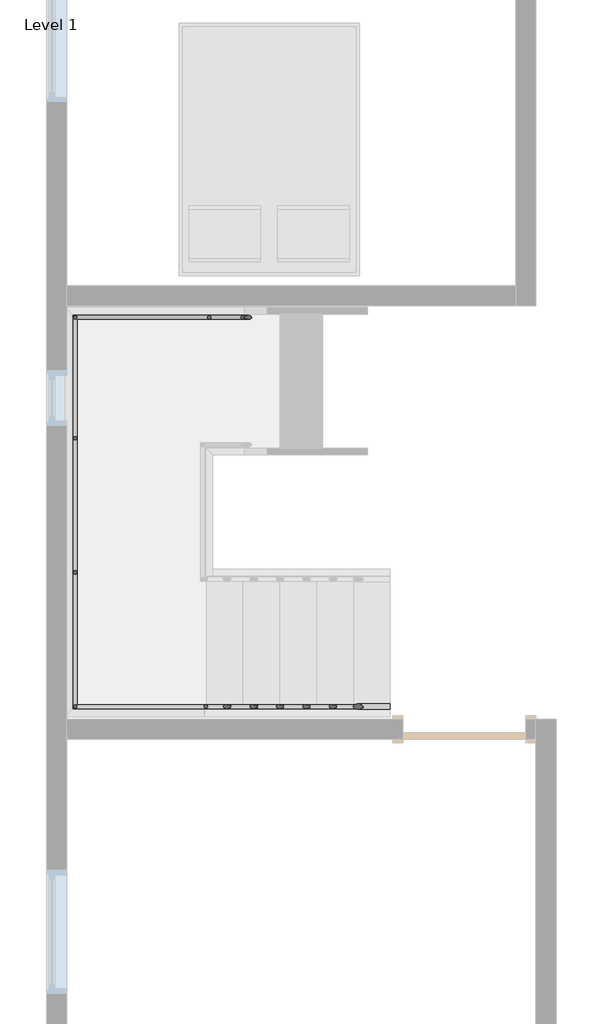
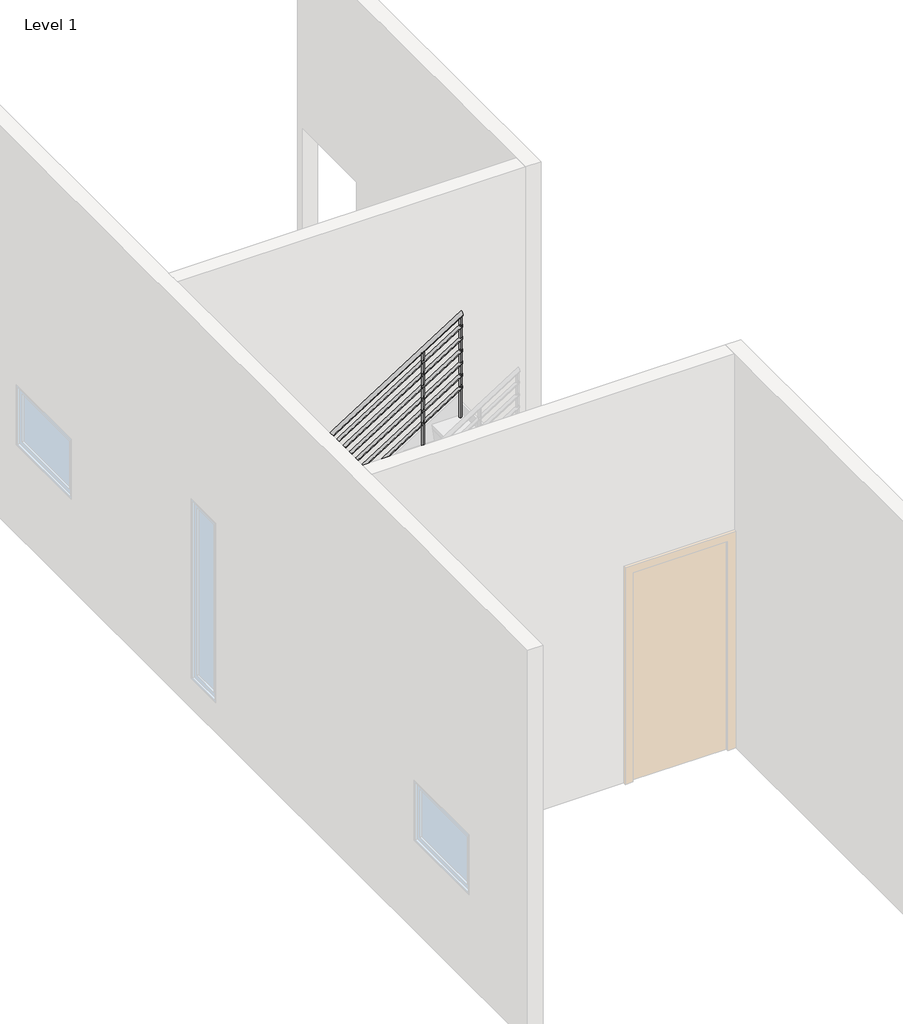
# One storey, part 3 of 4: 1 railing.
"""IFC4 building model written with IfcOpenShell, lengths in millimetres."""

from ifc_helpers import new_model, si_unit, point, frame, frame_2d, origin, place, context, project, spatial, circle_curve, ellipse_curve, trimmed, segment, composite_curve, outline, extrude, element, save
from ifc_brep_helpers import plane_surface, cylinder_surface, advanced_brep

model = new_model("IFC4")

# Units and contexts
model_context = context("Model", 3, world=origin())
ifc_project = project(units=[si_unit("LENGTHUNIT", "METRE", prefix="MILLI")], contexts=[model_context])

# Site, building, storey
site = spatial("IfcSite", under=ifc_project)
building = spatial("IfcBuilding", under=site)
storey = spatial("IfcBuildingStorey", under=building, Name="Level 1", Elevation=0.0)

# Railing
placement = place(None, origin())
element("IfcRailing", 1, ObjectType="900mm Pipe", at=placement, inside=storey, context=model_context, shape_type="SolidModel", body=[
    advanced_brep(
    [(-10589.1151057, 893.2798105, 1050.2491997), (-10589.1151057, 853.2798105, 1050.2491997), (-11969.9085587, 893.2798105, 1923.4782609), (-11969.9085587, 853.2798105, 1923.4782609), (-12918.740887, 893.2798105, 1923.4782609), (-12958.740887, 853.2798105, 1923.4782609), (-12918.740887, 3754.7656289, 1923.4782609), (-12958.740887, 3794.7656289, 1923.4782609), (-11683.3216527, 3754.7656289, 1923.4782609), (-11683.3216527, 3794.7656289, 1923.4782609), (-10314.1151057, 3754.7656289, 2789.3796345), (-10314.1151057, 3794.7656289, 2789.3796345)],
    [
        (0, 1, ellipse_curve(frame((-10589.1151057, 873.2798105, 1050.2491997), z_axis=(1.0, 0.0, 0.0), x_axis=(0.0, 0.0, -1.0)), 23.6638438, 20.0)),
        (1, 0, ellipse_curve(frame((-10589.1151057, 873.2798105, 1050.2491997), z_axis=(1.0, 0.0, 0.0), x_axis=(0.0, 0.0, -1.0)), 23.6638438, 20.0)),
        (0, 2),
        (2, 3, ellipse_curve(frame((-11969.9085587, 873.2798105, 1923.4782609), z_axis=(0.9605132043335071, 0.0, -0.27823440531497595), x_axis=(-0.2782344053149755, 0.0, -0.9605132043335074)), 20.822202, 20.0)),
        (3, 1),
        (3, 2, ellipse_curve(frame((-11969.9085587, 873.2798105, 1923.4782609), z_axis=(0.9605132043335071, 0.0, -0.27823440531497595), x_axis=(-0.2782344053149755, 0.0, -0.9605132043335074)), 20.822202, 20.0)),
        (2, 4),
        (4, 5, ellipse_curve(frame((-12938.740887, 873.2798105, 1923.4782609), z_axis=(0.7071067811865439, -0.7071067811865511, 0.0), x_axis=(0.7071067811865511, 0.7071067811865439, 0.0)), 28.2842712, 20.0)),
        (5, 3),
        (5, 4, ellipse_curve(frame((-12938.740887, 873.2798105, 1923.4782609), z_axis=(0.7071067811865439, -0.7071067811865511, 0.0), x_axis=(0.7071067811865511, 0.7071067811865439, 0.0)), 28.2842712, 20.0)),
        (4, 6),
        (6, 7, ellipse_curve(frame((-12938.740887, 3774.7656289, 1923.4782609), z_axis=(-0.7071067811865511, -0.7071067811865439, 0.0), x_axis=(0.7071067811865439, -0.7071067811865512, 0.0)), 28.2842712, 20.0)),
        (7, 5),
        (7, 6, ellipse_curve(frame((-12938.740887, 3774.7656289, 1923.4782609), z_axis=(-0.7071067811865511, -0.7071067811865439, 0.0), x_axis=(0.7071067811865439, -0.7071067811865512, 0.0)), 28.2842712, 20.0)),
        (6, 8),
        (8, 9, ellipse_curve(frame((-11683.3216527, 3774.7656289, 1923.4782609), z_axis=(-0.9605132043335074, 0.0, -0.2782344053149752), x_axis=(-0.2782344053149752, 0.0, 0.9605132043335074)), 20.822202, 20.0)),
        (9, 7),
        (9, 8, ellipse_curve(frame((-11683.3216527, 3774.7656289, 1923.4782609), z_axis=(-0.9605132043335074, 0.0, -0.2782344053149752), x_axis=(-0.2782344053149752, 0.0, 0.9605132043335074)), 20.822202, 20.0)),
        (10, 11, ellipse_curve(frame((-10314.1151057, 3774.7656289, 2789.3796345), z_axis=(1.0, 0.0, 0.0), x_axis=(0.0, 0.0, -1.0)), 23.6638438, 20.0)),
        (11, 10, ellipse_curve(frame((-10314.1151057, 3774.7656289, 2789.3796345), z_axis=(1.0, 0.0, 0.0), x_axis=(0.0, 0.0, -1.0)), 23.6638438, 20.0)),
        (8, 10),
        (11, 9),
    ],
    [
        plane_surface(frame((-10589.1151057, 873.2798105, 1073.9130435), z_axis=(1.0, 0.0, 0.0), x_axis=(0.0, -1.0, 0.0))),
        cylinder_surface(frame((-10599.8050185, 873.2798105, 1057.0096189), z_axis=(0.8451712313980434, 0.0, -0.5344956404098309), x_axis=(0.0, -1.0, 0.0)), 20.0),
        cylinder_surface(frame((-11964.1151057, 873.2798105, 1923.4782609), z_axis=(1.0, 0.0, 0.0), x_axis=(0.0, -1.0, 0.0)), 20.0),
        cylinder_surface(frame((-12938.740887, 873.2798105, 1923.4782609), z_axis=(0.0, -1.0, 0.0), x_axis=(-1.0, 0.0, 0.0)), 20.0),
        cylinder_surface(frame((-12938.740887, 3774.7656289, 1923.4782609), z_axis=(-1.0, 0.0, 0.0), x_axis=(0.0, 1.0, 0.0)), 20.0),
        plane_surface(frame((-10314.1151057, 3774.7656289, 2813.0434783), z_axis=(1.0, 0.0, 0.0), x_axis=(0.0, 1.0, 0.0))),
        cylinder_surface(frame((-11678.4251929, 3774.7656289, 1926.5748362), z_axis=(-0.8451712313980442, 0.0, -0.5344956404098294), x_axis=(0.0, 1.0, 0.0)), 20.0),
    ],
    [
        (0, [[1, 2]]),
        (1, [[-1, 3, 4, 5]]),
        (1, [[-2, -5, 6, -3]]),
        (2, [[-4, 7, 8, 9]]),
        (2, [[-6, -9, 10, -7]]),
        (3, [[-8, 11, 12, 13]]),
        (3, [[-10, -13, 14, -11]]),
        (4, [[-12, 15, 16, 17]]),
        (4, [[-14, -17, 18, -15]]),
        (5, [[19, 20]]),
        (6, [[-16, 21, -20, 22]]),
        (6, [[-18, -22, -19, -21]]),
    ],
),
    advanced_brep(
    [(-10589.1151057, 888.2798105, 931.1651606), (-10589.1151057, 858.2798105, 931.1651606), (-11968.4601955, 888.2798105, 1803.4782609), (-11968.4601955, 858.2798105, 1803.4782609), (-12923.740887, 888.2798105, 1803.4782609), (-12953.740887, 858.2798105, 1803.4782609), (-12923.740887, 3759.7656289, 1803.4782609), (-12953.740887, 3789.7656289, 1803.4782609), (-11684.7700159, 3759.7656289, 1803.4782609), (-11684.7700159, 3789.7656289, 1803.4782609), (-10314.1151057, 3759.7656289, 2670.2955954), (-10314.1151057, 3789.7656289, 2670.2955954)],
    [
        (0, 1, ellipse_curve(frame((-10589.1151057, 873.2798105, 931.1651606), z_axis=(1.0, 0.0, 0.0), x_axis=(0.0, 0.0, -1.0)), 17.7478828, 15.0)),
        (1, 0, ellipse_curve(frame((-10589.1151057, 873.2798105, 931.1651606), z_axis=(1.0, 0.0, 0.0), x_axis=(0.0, 0.0, -1.0)), 17.7478828, 15.0)),
        (0, 2),
        (2, 3, ellipse_curve(frame((-11968.4601955, 873.2798105, 1803.4782609), z_axis=(0.9605132043335071, 0.0, -0.2782344053149759), x_axis=(-0.27823440531497556, 0.0, -0.9605132043335073)), 15.6166515, 15.0)),
        (3, 1),
        (3, 2, ellipse_curve(frame((-11968.4601955, 873.2798105, 1803.4782609), z_axis=(0.9605132043335071, 0.0, -0.2782344053149759), x_axis=(-0.27823440531497556, 0.0, -0.9605132043335073)), 15.6166515, 15.0)),
        (2, 4),
        (4, 5, ellipse_curve(frame((-12938.740887, 873.2798105, 1803.4782609), z_axis=(0.7071067811865439, -0.7071067811865511, 0.0), x_axis=(0.7071067811865511, 0.7071067811865439, 0.0)), 21.2132034, 15.0)),
        (5, 3),
        (5, 4, ellipse_curve(frame((-12938.740887, 873.2798105, 1803.4782609), z_axis=(0.7071067811865439, -0.7071067811865511, 0.0), x_axis=(0.7071067811865511, 0.7071067811865439, 0.0)), 21.2132034, 15.0)),
        (4, 6),
        (6, 7, ellipse_curve(frame((-12938.740887, 3774.7656289, 1803.4782609), z_axis=(-0.7071067811865511, -0.7071067811865439, 0.0), x_axis=(0.7071067811865439, -0.7071067811865512, 0.0)), 21.2132034, 15.0)),
        (7, 5),
        (7, 6, ellipse_curve(frame((-12938.740887, 3774.7656289, 1803.4782609), z_axis=(-0.7071067811865511, -0.7071067811865439, 0.0), x_axis=(0.7071067811865439, -0.7071067811865512, 0.0)), 21.2132034, 15.0)),
        (6, 8),
        (8, 9, ellipse_curve(frame((-11684.7700159, 3774.7656289, 1803.4782609), z_axis=(-0.9605132043335073, 0.0, -0.2782344053149753), x_axis=(-0.2782344053149759, 0.0, 0.9605132043335072)), 15.6166515, 15.0)),
        (9, 7),
        (9, 8, ellipse_curve(frame((-11684.7700159, 3774.7656289, 1803.4782609), z_axis=(-0.9605132043335073, 0.0, -0.2782344053149753), x_axis=(-0.2782344053149759, 0.0, 0.9605132043335072)), 15.6166515, 15.0)),
        (10, 11, ellipse_curve(frame((-10314.1151057, 3774.7656289, 2670.2955954), z_axis=(1.0, 0.0, 0.0), x_axis=(0.0, 0.0, -1.0)), 17.7478828, 15.0)),
        (11, 10, ellipse_curve(frame((-10314.1151057, 3774.7656289, 2670.2955954), z_axis=(1.0, 0.0, 0.0), x_axis=(0.0, 0.0, -1.0)), 17.7478828, 15.0)),
        (8, 10),
        (11, 9),
    ],
    [
        plane_surface(frame((-10589.1151057, 873.2798105, 948.9130435), z_axis=(1.0, 0.0, 0.0), x_axis=(0.0, -1.0, 0.0))),
        cylinder_surface(frame((-10597.1325403, 873.2798105, 936.235475), z_axis=(0.8451712313980434, 0.0, -0.5344956404098308), x_axis=(0.0, -1.0, 0.0)), 15.0),
        cylinder_surface(frame((-11964.1151057, 873.2798105, 1803.4782609), z_axis=(1.0, 0.0, 0.0), x_axis=(0.0, -1.0, 0.0)), 15.0),
        cylinder_surface(frame((-12938.740887, 873.2798105, 1803.4782609), z_axis=(0.0, -1.0, 0.0), x_axis=(-1.0, 0.0, 0.0)), 15.0),
        cylinder_surface(frame((-12938.740887, 3774.7656289, 1803.4782609), z_axis=(-1.0, 0.0, 0.0), x_axis=(0.0, 1.0, 0.0)), 15.0),
        plane_surface(frame((-10314.1151057, 3774.7656289, 2688.0434783), z_axis=(1.0, 0.0, 0.0), x_axis=(0.0, 1.0, 0.0))),
        cylinder_surface(frame((-11681.0976711, 3774.7656289, 1805.8006924), z_axis=(-0.845171231398044, 0.0, -0.5344956404098297), x_axis=(0.0, 1.0, 0.0)), 15.0),
    ],
    [
        (0, [[1, 2]]),
        (1, [[-1, 3, 4, 5]]),
        (1, [[-2, -5, 6, -3]]),
        (2, [[-4, 7, 8, 9]]),
        (2, [[-6, -9, 10, -7]]),
        (3, [[-8, 11, 12, 13]]),
        (3, [[-10, -13, 14, -11]]),
        (4, [[-12, 15, 16, 17]]),
        (4, [[-14, -17, 18, -15]]),
        (5, [[19, 20]]),
        (6, [[-16, 21, -20, 22]]),
        (6, [[-18, -22, -19, -21]]),
    ],
),
    advanced_brep(
    [(-10589.1151057, 888.2798105, 806.1651606), (-10589.1151057, 858.2798105, 806.1651606), (-11968.4601955, 888.2798105, 1678.4782609), (-11968.4601955, 858.2798105, 1678.4782609), (-12923.740887, 888.2798105, 1678.4782609), (-12953.740887, 858.2798105, 1678.4782609), (-12923.740887, 3759.7656289, 1678.4782609), (-12953.740887, 3789.7656289, 1678.4782609), (-11684.7700159, 3759.7656289, 1678.4782609), (-11684.7700159, 3789.7656289, 1678.4782609), (-10314.1151057, 3759.7656289, 2545.2955954), (-10314.1151057, 3789.7656289, 2545.2955954)],
    [
        (0, 1, ellipse_curve(frame((-10589.1151057, 873.2798105, 806.1651606), z_axis=(1.0, 0.0, 0.0), x_axis=(0.0, 0.0, -1.0)), 17.7478828, 15.0)),
        (1, 0, ellipse_curve(frame((-10589.1151057, 873.2798105, 806.1651606), z_axis=(1.0, 0.0, 0.0), x_axis=(0.0, 0.0, -1.0)), 17.7478828, 15.0)),
        (0, 2),
        (2, 3, ellipse_curve(frame((-11968.4601955, 873.2798105, 1678.4782609), z_axis=(0.9605132043335071, 0.0, -0.2782344053149759), x_axis=(-0.27823440531497556, 0.0, -0.9605132043335073)), 15.6166515, 15.0)),
        (3, 1),
        (3, 2, ellipse_curve(frame((-11968.4601955, 873.2798105, 1678.4782609), z_axis=(0.9605132043335071, 0.0, -0.2782344053149759), x_axis=(-0.27823440531497556, 0.0, -0.9605132043335073)), 15.6166515, 15.0)),
        (2, 4),
        (4, 5, ellipse_curve(frame((-12938.740887, 873.2798105, 1678.4782609), z_axis=(0.7071067811865439, -0.7071067811865511, 0.0), x_axis=(0.7071067811865511, 0.7071067811865439, 0.0)), 21.2132034, 15.0)),
        (5, 3),
        (5, 4, ellipse_curve(frame((-12938.740887, 873.2798105, 1678.4782609), z_axis=(0.7071067811865439, -0.7071067811865511, 0.0), x_axis=(0.7071067811865511, 0.7071067811865439, 0.0)), 21.2132034, 15.0)),
        (4, 6),
        (6, 7, ellipse_curve(frame((-12938.740887, 3774.7656289, 1678.4782609), z_axis=(-0.7071067811865511, -0.7071067811865439, 0.0), x_axis=(0.7071067811865439, -0.7071067811865512, 0.0)), 21.2132034, 15.0)),
        (7, 5),
        (7, 6, ellipse_curve(frame((-12938.740887, 3774.7656289, 1678.4782609), z_axis=(-0.7071067811865511, -0.7071067811865439, 0.0), x_axis=(0.7071067811865439, -0.7071067811865512, 0.0)), 21.2132034, 15.0)),
        (6, 8),
        (8, 9, ellipse_curve(frame((-11684.7700159, 3774.7656289, 1678.4782609), z_axis=(-0.9605132043335073, 0.0, -0.27823440531497523), x_axis=(-0.27823440531497595, 0.0, 0.9605132043335072)), 15.6166515, 15.0)),
        (9, 7),
        (9, 8, ellipse_curve(frame((-11684.7700159, 3774.7656289, 1678.4782609), z_axis=(-0.9605132043335073, 0.0, -0.27823440531497523), x_axis=(-0.27823440531497595, 0.0, 0.9605132043335072)), 15.6166515, 15.0)),
        (10, 11, ellipse_curve(frame((-10314.1151057, 3774.7656289, 2545.2955954), z_axis=(1.0, 0.0, 0.0), x_axis=(0.0, 0.0, -1.0)), 17.7478828, 15.0)),
        (11, 10, ellipse_curve(frame((-10314.1151057, 3774.7656289, 2545.2955954), z_axis=(1.0, 0.0, 0.0), x_axis=(0.0, 0.0, -1.0)), 17.7478828, 15.0)),
        (8, 10),
        (11, 9),
    ],
    [
        plane_surface(frame((-10589.1151057, 873.2798105, 823.9130435), z_axis=(1.0, 0.0, 0.0), x_axis=(0.0, -1.0, 0.0))),
        cylinder_surface(frame((-10597.1325403, 873.2798105, 811.235475), z_axis=(0.8451712313980434, 0.0, -0.5344956404098308), x_axis=(0.0, -1.0, 0.0)), 15.0),
        cylinder_surface(frame((-11964.1151057, 873.2798105, 1678.4782609), z_axis=(1.0, 0.0, 0.0), x_axis=(0.0, -1.0, 0.0)), 15.0),
        cylinder_surface(frame((-12938.740887, 873.2798105, 1678.4782609), z_axis=(0.0, -1.0, 0.0), x_axis=(-1.0, 0.0, 0.0)), 15.0),
        cylinder_surface(frame((-12938.740887, 3774.7656289, 1678.4782609), z_axis=(-1.0, 0.0, 0.0), x_axis=(0.0, 1.0, 0.0)), 15.0),
        plane_surface(frame((-10314.1151057, 3774.7656289, 2563.0434783), z_axis=(1.0, 0.0, 0.0), x_axis=(0.0, 1.0, 0.0))),
        cylinder_surface(frame((-11681.0976711, 3774.7656289, 1680.8006924), z_axis=(-0.8451712313980441, 0.0, -0.5344956404098296), x_axis=(0.0, 1.0, 0.0)), 15.0),
    ],
    [
        (0, [[1, 2]]),
        (1, [[-1, 3, 4, 5]]),
        (1, [[-2, -5, 6, -3]]),
        (2, [[-4, 7, 8, 9]]),
        (2, [[-6, -9, 10, -7]]),
        (3, [[-8, 11, 12, 13]]),
        (3, [[-10, -13, 14, -11]]),
        (4, [[-12, 15, 16, 17]]),
        (4, [[-14, -17, 18, -15]]),
        (5, [[19, 20]]),
        (6, [[-16, 21, -20, 22]]),
        (6, [[-18, -22, -19, -21]]),
    ],
),
    advanced_brep(
    [(-10589.1151057, 888.2798105, 681.1651606), (-10589.1151057, 858.2798105, 681.1651606), (-11968.4601955, 888.2798105, 1553.4782609), (-11968.4601955, 858.2798105, 1553.4782609), (-12923.740887, 888.2798105, 1553.4782609), (-12953.740887, 858.2798105, 1553.4782609), (-12923.740887, 3759.7656289, 1553.4782609), (-12953.740887, 3789.7656289, 1553.4782609), (-11684.7700159, 3759.7656289, 1553.4782609), (-11684.7700159, 3789.7656289, 1553.4782609), (-10314.1151057, 3759.7656289, 2420.2955954), (-10314.1151057, 3789.7656289, 2420.2955954)],
    [
        (0, 1, ellipse_curve(frame((-10589.1151057, 873.2798105, 681.1651606), z_axis=(1.0, 0.0, 0.0), x_axis=(0.0, 0.0, -1.0)), 17.7478828, 15.0)),
        (1, 0, ellipse_curve(frame((-10589.1151057, 873.2798105, 681.1651606), z_axis=(1.0, 0.0, 0.0), x_axis=(0.0, 0.0, -1.0)), 17.7478828, 15.0)),
        (0, 2),
        (2, 3, ellipse_curve(frame((-11968.4601955, 873.2798105, 1553.4782609), z_axis=(0.9605132043335071, 0.0, -0.2782344053149759), x_axis=(-0.27823440531497556, 0.0, -0.9605132043335073)), 15.6166515, 15.0)),
        (3, 1),
        (3, 2, ellipse_curve(frame((-11968.4601955, 873.2798105, 1553.4782609), z_axis=(0.9605132043335071, 0.0, -0.2782344053149759), x_axis=(-0.27823440531497556, 0.0, -0.9605132043335073)), 15.6166515, 15.0)),
        (2, 4),
        (4, 5, ellipse_curve(frame((-12938.740887, 873.2798105, 1553.4782609), z_axis=(0.7071067811865439, -0.7071067811865511, 0.0), x_axis=(0.7071067811865511, 0.7071067811865439, 0.0)), 21.2132034, 15.0)),
        (5, 3),
        (5, 4, ellipse_curve(frame((-12938.740887, 873.2798105, 1553.4782609), z_axis=(0.7071067811865439, -0.7071067811865511, 0.0), x_axis=(0.7071067811865511, 0.7071067811865439, 0.0)), 21.2132034, 15.0)),
        (4, 6),
        (6, 7, ellipse_curve(frame((-12938.740887, 3774.7656289, 1553.4782609), z_axis=(-0.7071067811865511, -0.7071067811865439, 0.0), x_axis=(0.7071067811865439, -0.7071067811865512, 0.0)), 21.2132034, 15.0)),
        (7, 5),
        (7, 6, ellipse_curve(frame((-12938.740887, 3774.7656289, 1553.4782609), z_axis=(-0.7071067811865511, -0.7071067811865439, 0.0), x_axis=(0.7071067811865439, -0.7071067811865512, 0.0)), 21.2132034, 15.0)),
        (6, 8),
        (8, 9, ellipse_curve(frame((-11684.7700159, 3774.7656289, 1553.4782609), z_axis=(-0.9605132043335073, 0.0, -0.2782344053149753), x_axis=(-0.2782344053149759, 0.0, 0.9605132043335072)), 15.6166515, 15.0)),
        (9, 7),
        (9, 8, ellipse_curve(frame((-11684.7700159, 3774.7656289, 1553.4782609), z_axis=(-0.9605132043335073, 0.0, -0.2782344053149753), x_axis=(-0.2782344053149759, 0.0, 0.9605132043335072)), 15.6166515, 15.0)),
        (10, 11, ellipse_curve(frame((-10314.1151057, 3774.7656289, 2420.2955954), z_axis=(1.0, 0.0, 0.0), x_axis=(0.0, 0.0, -1.0)), 17.7478828, 15.0)),
        (11, 10, ellipse_curve(frame((-10314.1151057, 3774.7656289, 2420.2955954), z_axis=(1.0, 0.0, 0.0), x_axis=(0.0, 0.0, -1.0)), 17.7478828, 15.0)),
        (8, 10),
        (11, 9),
    ],
    [
        plane_surface(frame((-10589.1151057, 873.2798105, 698.9130435), z_axis=(1.0, 0.0, 0.0), x_axis=(0.0, -1.0, 0.0))),
        cylinder_surface(frame((-10597.1325403, 873.2798105, 686.235475), z_axis=(0.8451712313980434, 0.0, -0.5344956404098308), x_axis=(0.0, -1.0, 0.0)), 15.0),
        cylinder_surface(frame((-11964.1151057, 873.2798105, 1553.4782609), z_axis=(1.0, 0.0, 0.0), x_axis=(0.0, -1.0, 0.0)), 15.0),
        cylinder_surface(frame((-12938.740887, 873.2798105, 1553.4782609), z_axis=(0.0, -1.0, 0.0), x_axis=(-1.0, 0.0, 0.0)), 15.0),
        cylinder_surface(frame((-12938.740887, 3774.7656289, 1553.4782609), z_axis=(-1.0, 0.0, 0.0), x_axis=(0.0, 1.0, 0.0)), 15.0),
        plane_surface(frame((-10314.1151057, 3774.7656289, 2438.0434783), z_axis=(1.0, 0.0, 0.0), x_axis=(0.0, 1.0, 0.0))),
        cylinder_surface(frame((-11681.0976711, 3774.7656289, 1555.8006924), z_axis=(-0.845171231398044, 0.0, -0.5344956404098297), x_axis=(0.0, 1.0, 0.0)), 15.0),
    ],
    [
        (0, [[1, 2]]),
        (1, [[-1, 3, 4, 5]]),
        (1, [[-2, -5, 6, -3]]),
        (2, [[-4, 7, 8, 9]]),
        (2, [[-6, -9, 10, -7]]),
        (3, [[-8, 11, 12, 13]]),
        (3, [[-10, -13, 14, -11]]),
        (4, [[-12, 15, 16, 17]]),
        (4, [[-14, -17, 18, -15]]),
        (5, [[19, 20]]),
        (6, [[-16, 21, -20, 22]]),
        (6, [[-18, -22, -19, -21]]),
    ],
),
    advanced_brep(
    [(-10589.1151057, 888.2798105, 556.1651606), (-10589.1151057, 858.2798105, 556.1651606), (-11968.4601955, 888.2798105, 1428.4782609), (-11968.4601955, 858.2798105, 1428.4782609), (-12923.740887, 888.2798105, 1428.4782609), (-12953.740887, 858.2798105, 1428.4782609), (-12923.740887, 3759.7656289, 1428.4782609), (-12953.740887, 3789.7656289, 1428.4782609), (-11684.7700159, 3759.7656289, 1428.4782609), (-11684.7700159, 3789.7656289, 1428.4782609), (-10314.1151057, 3759.7656289, 2295.2955954), (-10314.1151057, 3789.7656289, 2295.2955954)],
    [
        (0, 1, ellipse_curve(frame((-10589.1151057, 873.2798105, 556.1651606), z_axis=(1.0, 0.0, 0.0), x_axis=(0.0, 0.0, -1.0)), 17.7478828, 15.0)),
        (1, 0, ellipse_curve(frame((-10589.1151057, 873.2798105, 556.1651606), z_axis=(1.0, 0.0, 0.0), x_axis=(0.0, 0.0, -1.0)), 17.7478828, 15.0)),
        (0, 2),
        (2, 3, ellipse_curve(frame((-11968.4601955, 873.2798105, 1428.4782609), z_axis=(0.9605132043335071, 0.0, -0.2782344053149759), x_axis=(-0.27823440531497556, 0.0, -0.9605132043335073)), 15.6166515, 15.0)),
        (3, 1),
        (3, 2, ellipse_curve(frame((-11968.4601955, 873.2798105, 1428.4782609), z_axis=(0.9605132043335071, 0.0, -0.2782344053149759), x_axis=(-0.27823440531497556, 0.0, -0.9605132043335073)), 15.6166515, 15.0)),
        (2, 4),
        (4, 5, ellipse_curve(frame((-12938.740887, 873.2798105, 1428.4782609), z_axis=(0.7071067811865439, -0.7071067811865511, 0.0), x_axis=(0.7071067811865511, 0.7071067811865439, 0.0)), 21.2132034, 15.0)),
        (5, 3),
        (5, 4, ellipse_curve(frame((-12938.740887, 873.2798105, 1428.4782609), z_axis=(0.7071067811865439, -0.7071067811865511, 0.0), x_axis=(0.7071067811865511, 0.7071067811865439, 0.0)), 21.2132034, 15.0)),
        (4, 6),
        (6, 7, ellipse_curve(frame((-12938.740887, 3774.7656289, 1428.4782609), z_axis=(-0.7071067811865511, -0.7071067811865439, 0.0), x_axis=(0.7071067811865439, -0.7071067811865512, 0.0)), 21.2132034, 15.0)),
        (7, 5),
        (7, 6, ellipse_curve(frame((-12938.740887, 3774.7656289, 1428.4782609), z_axis=(-0.7071067811865511, -0.7071067811865439, 0.0), x_axis=(0.7071067811865439, -0.7071067811865512, 0.0)), 21.2132034, 15.0)),
        (6, 8),
        (8, 9, ellipse_curve(frame((-11684.7700159, 3774.7656289, 1428.4782609), z_axis=(-0.9605132043335073, 0.0, -0.2782344053149753), x_axis=(-0.2782344053149759, 0.0, 0.9605132043335072)), 15.6166515, 15.0)),
        (9, 7),
        (9, 8, ellipse_curve(frame((-11684.7700159, 3774.7656289, 1428.4782609), z_axis=(-0.9605132043335073, 0.0, -0.2782344053149753), x_axis=(-0.2782344053149759, 0.0, 0.9605132043335072)), 15.6166515, 15.0)),
        (10, 11, ellipse_curve(frame((-10314.1151057, 3774.7656289, 2295.2955954), z_axis=(1.0, 0.0, 0.0), x_axis=(0.0, 0.0, -1.0)), 17.7478828, 15.0)),
        (11, 10, ellipse_curve(frame((-10314.1151057, 3774.7656289, 2295.2955954), z_axis=(1.0, 0.0, 0.0), x_axis=(0.0, 0.0, -1.0)), 17.7478828, 15.0)),
        (8, 10),
        (11, 9),
    ],
    [
        plane_surface(frame((-10589.1151057, 873.2798105, 573.9130435), z_axis=(1.0, 0.0, 0.0), x_axis=(0.0, -1.0, 0.0))),
        cylinder_surface(frame((-10597.1325403, 873.2798105, 561.235475), z_axis=(0.8451712313980434, 0.0, -0.5344956404098308), x_axis=(0.0, -1.0, 0.0)), 15.0),
        cylinder_surface(frame((-11964.1151057, 873.2798105, 1428.4782609), z_axis=(1.0, 0.0, 0.0), x_axis=(0.0, -1.0, 0.0)), 15.0),
        cylinder_surface(frame((-12938.740887, 873.2798105, 1428.4782609), z_axis=(0.0, -1.0, 0.0), x_axis=(-1.0, 0.0, 0.0)), 15.0),
        cylinder_surface(frame((-12938.740887, 3774.7656289, 1428.4782609), z_axis=(-1.0, 0.0, 0.0), x_axis=(0.0, 1.0, 0.0)), 15.0),
        plane_surface(frame((-10314.1151057, 3774.7656289, 2313.0434783), z_axis=(1.0, 0.0, 0.0), x_axis=(0.0, 1.0, 0.0))),
        cylinder_surface(frame((-11681.0976711, 3774.7656289, 1430.8006924), z_axis=(-0.845171231398044, 0.0, -0.5344956404098297), x_axis=(0.0, 1.0, 0.0)), 15.0),
    ],
    [
        (0, [[1, 2]]),
        (1, [[-1, 3, 4, 5]]),
        (1, [[-2, -5, 6, -3]]),
        (2, [[-4, 7, 8, 9]]),
        (2, [[-6, -9, 10, -7]]),
        (3, [[-8, 11, 12, 13]]),
        (3, [[-10, -13, 14, -11]]),
        (4, [[-12, 15, 16, 17]]),
        (4, [[-14, -17, 18, -15]]),
        (5, [[19, 20]]),
        (6, [[-16, 21, -20, 22]]),
        (6, [[-18, -22, -19, -21]]),
    ],
),
    advanced_brep(
    [(-10589.1151057, 888.2798105, 431.1651606), (-10589.1151057, 858.2798105, 431.1651606), (-11968.4601955, 888.2798105, 1303.4782609), (-11968.4601955, 858.2798105, 1303.4782609), (-12923.740887, 888.2798105, 1303.4782609), (-12953.740887, 858.2798105, 1303.4782609), (-12923.740887, 3759.7656289, 1303.4782609), (-12953.740887, 3789.7656289, 1303.4782609), (-11684.7700159, 3759.7656289, 1303.4782609), (-11684.7700159, 3789.7656289, 1303.4782609), (-10314.1151057, 3759.7656289, 2170.2955954), (-10314.1151057, 3789.7656289, 2170.2955954)],
    [
        (0, 1, ellipse_curve(frame((-10589.1151057, 873.2798105, 431.1651606), z_axis=(1.0, 0.0, 0.0), x_axis=(0.0, 0.0, -1.0)), 17.7478828, 15.0)),
        (1, 0, ellipse_curve(frame((-10589.1151057, 873.2798105, 431.1651606), z_axis=(1.0, 0.0, 0.0), x_axis=(0.0, 0.0, -1.0)), 17.7478828, 15.0)),
        (0, 2),
        (2, 3, ellipse_curve(frame((-11968.4601955, 873.2798105, 1303.4782609), z_axis=(0.9605132043335071, 0.0, -0.2782344053149759), x_axis=(-0.27823440531497556, 0.0, -0.9605132043335073)), 15.6166515, 15.0)),
        (3, 1),
        (3, 2, ellipse_curve(frame((-11968.4601955, 873.2798105, 1303.4782609), z_axis=(0.9605132043335071, 0.0, -0.2782344053149759), x_axis=(-0.27823440531497556, 0.0, -0.9605132043335073)), 15.6166515, 15.0)),
        (2, 4),
        (4, 5, ellipse_curve(frame((-12938.740887, 873.2798105, 1303.4782609), z_axis=(0.7071067811865439, -0.7071067811865511, 0.0), x_axis=(0.7071067811865511, 0.7071067811865439, 0.0)), 21.2132034, 15.0)),
        (5, 3),
        (5, 4, ellipse_curve(frame((-12938.740887, 873.2798105, 1303.4782609), z_axis=(0.7071067811865439, -0.7071067811865511, 0.0), x_axis=(0.7071067811865511, 0.7071067811865439, 0.0)), 21.2132034, 15.0)),
        (4, 6),
        (6, 7, ellipse_curve(frame((-12938.740887, 3774.7656289, 1303.4782609), z_axis=(-0.7071067811865511, -0.7071067811865439, 0.0), x_axis=(0.7071067811865439, -0.7071067811865512, 0.0)), 21.2132034, 15.0)),
        (7, 5),
        (7, 6, ellipse_curve(frame((-12938.740887, 3774.7656289, 1303.4782609), z_axis=(-0.7071067811865511, -0.7071067811865439, 0.0), x_axis=(0.7071067811865439, -0.7071067811865512, 0.0)), 21.2132034, 15.0)),
        (6, 8),
        (8, 9, ellipse_curve(frame((-11684.7700159, 3774.7656289, 1303.4782609), z_axis=(-0.9605132043335073, 0.0, -0.2782344053149753), x_axis=(-0.2782344053149759, 0.0, 0.9605132043335072)), 15.6166515, 15.0)),
        (9, 7),
        (9, 8, ellipse_curve(frame((-11684.7700159, 3774.7656289, 1303.4782609), z_axis=(-0.9605132043335073, 0.0, -0.2782344053149753), x_axis=(-0.2782344053149759, 0.0, 0.9605132043335072)), 15.6166515, 15.0)),
        (10, 11, ellipse_curve(frame((-10314.1151057, 3774.7656289, 2170.2955954), z_axis=(1.0, 0.0, 0.0), x_axis=(0.0, 0.0, -1.0)), 17.7478828, 15.0)),
        (11, 10, ellipse_curve(frame((-10314.1151057, 3774.7656289, 2170.2955954), z_axis=(1.0, 0.0, 0.0), x_axis=(0.0, 0.0, -1.0)), 17.7478828, 15.0)),
        (8, 10),
        (11, 9),
    ],
    [
        plane_surface(frame((-10589.1151057, 873.2798105, 448.9130435), z_axis=(1.0, 0.0, 0.0), x_axis=(0.0, -1.0, 0.0))),
        cylinder_surface(frame((-10597.1325403, 873.2798105, 436.235475), z_axis=(0.8451712313980434, 0.0, -0.5344956404098308), x_axis=(0.0, -1.0, 0.0)), 15.0),
        cylinder_surface(frame((-11964.1151057, 873.2798105, 1303.4782609), z_axis=(1.0, 0.0, 0.0), x_axis=(0.0, -1.0, 0.0)), 15.0),
        cylinder_surface(frame((-12938.740887, 873.2798105, 1303.4782609), z_axis=(0.0, -1.0, 0.0), x_axis=(-1.0, 0.0, 0.0)), 15.0),
        cylinder_surface(frame((-12938.740887, 3774.7656289, 1303.4782609), z_axis=(-1.0, 0.0, 0.0), x_axis=(0.0, 1.0, 0.0)), 15.0),
        plane_surface(frame((-10314.1151057, 3774.7656289, 2188.0434783), z_axis=(1.0, 0.0, 0.0), x_axis=(0.0, 1.0, 0.0))),
        cylinder_surface(frame((-11681.0976711, 3774.7656289, 1305.8006924), z_axis=(-0.845171231398044, 0.0, -0.5344956404098297), x_axis=(0.0, 1.0, 0.0)), 15.0),
    ],
    [
        (0, [[1, 2]]),
        (1, [[-1, 3, 4, 5]]),
        (1, [[-2, -5, 6, -3]]),
        (2, [[-4, 7, 8, 9]]),
        (2, [[-6, -9, 10, -7]]),
        (3, [[-8, 11, 12, 13]]),
        (3, [[-10, -13, 14, -11]]),
        (4, [[-12, 15, 16, 17]]),
        (4, [[-14, -17, 18, -15]]),
        (5, [[19, 20]]),
        (6, [[-16, 21, -20, 22]]),
        (6, [[-18, -22, -19, -21]]),
    ],
),
    advanced_brep(
    [(-10589.1151057, 888.2798105, 306.1651606), (-10589.1151057, 858.2798105, 306.1651606), (-11968.4601955, 888.2798105, 1178.4782609), (-11968.4601955, 858.2798105, 1178.4782609), (-12923.740887, 888.2798105, 1178.4782609), (-12953.740887, 858.2798105, 1178.4782609), (-12923.740887, 3759.7656289, 1178.4782609), (-12953.740887, 3789.7656289, 1178.4782609), (-11684.7700159, 3759.7656289, 1178.4782609), (-11684.7700159, 3789.7656289, 1178.4782609), (-10314.1151057, 3759.7656289, 2045.2955954), (-10314.1151057, 3789.7656289, 2045.2955954)],
    [
        (0, 1, ellipse_curve(frame((-10589.1151057, 873.2798105, 306.1651606), z_axis=(1.0, 0.0, 0.0), x_axis=(0.0, 0.0, -1.0)), 17.7478828, 15.0)),
        (1, 0, ellipse_curve(frame((-10589.1151057, 873.2798105, 306.1651606), z_axis=(1.0, 0.0, 0.0), x_axis=(0.0, 0.0, -1.0)), 17.7478828, 15.0)),
        (0, 2),
        (2, 3, ellipse_curve(frame((-11968.4601955, 873.2798105, 1178.4782609), z_axis=(0.9605132043335071, 0.0, -0.2782344053149759), x_axis=(-0.27823440531497556, 0.0, -0.9605132043335073)), 15.6166515, 15.0)),
        (3, 1),
        (3, 2, ellipse_curve(frame((-11968.4601955, 873.2798105, 1178.4782609), z_axis=(0.9605132043335071, 0.0, -0.2782344053149759), x_axis=(-0.27823440531497556, 0.0, -0.9605132043335073)), 15.6166515, 15.0)),
        (2, 4),
        (4, 5, ellipse_curve(frame((-12938.740887, 873.2798105, 1178.4782609), z_axis=(0.7071067811865439, -0.7071067811865511, 0.0), x_axis=(0.7071067811865511, 0.7071067811865439, 0.0)), 21.2132034, 15.0)),
        (5, 3),
        (5, 4, ellipse_curve(frame((-12938.740887, 873.2798105, 1178.4782609), z_axis=(0.7071067811865439, -0.7071067811865511, 0.0), x_axis=(0.7071067811865511, 0.7071067811865439, 0.0)), 21.2132034, 15.0)),
        (4, 6),
        (6, 7, ellipse_curve(frame((-12938.740887, 3774.7656289, 1178.4782609), z_axis=(-0.7071067811865511, -0.7071067811865439, 0.0), x_axis=(0.7071067811865439, -0.7071067811865512, 0.0)), 21.2132034, 15.0)),
        (7, 5),
        (7, 6, ellipse_curve(frame((-12938.740887, 3774.7656289, 1178.4782609), z_axis=(-0.7071067811865511, -0.7071067811865439, 0.0), x_axis=(0.7071067811865439, -0.7071067811865512, 0.0)), 21.2132034, 15.0)),
        (6, 8),
        (8, 9, ellipse_curve(frame((-11684.7700159, 3774.7656289, 1178.4782609), z_axis=(-0.9605132043335073, 0.0, -0.2782344053149753), x_axis=(-0.2782344053149759, 0.0, 0.9605132043335072)), 15.6166515, 15.0)),
        (9, 7),
        (9, 8, ellipse_curve(frame((-11684.7700159, 3774.7656289, 1178.4782609), z_axis=(-0.9605132043335073, 0.0, -0.2782344053149753), x_axis=(-0.2782344053149759, 0.0, 0.9605132043335072)), 15.6166515, 15.0)),
        (10, 11, ellipse_curve(frame((-10314.1151057, 3774.7656289, 2045.2955954), z_axis=(1.0, 0.0, 0.0), x_axis=(0.0, 0.0, -1.0)), 17.7478828, 15.0)),
        (11, 10, ellipse_curve(frame((-10314.1151057, 3774.7656289, 2045.2955954), z_axis=(1.0, 0.0, 0.0), x_axis=(0.0, 0.0, -1.0)), 17.7478828, 15.0)),
        (8, 10),
        (11, 9),
    ],
    [
        plane_surface(frame((-10589.1151057, 873.2798105, 323.9130435), z_axis=(1.0, 0.0, 0.0), x_axis=(0.0, -1.0, 0.0))),
        cylinder_surface(frame((-10597.1325403, 873.2798105, 311.235475), z_axis=(0.8451712313980434, 0.0, -0.5344956404098308), x_axis=(0.0, -1.0, 0.0)), 15.0),
        cylinder_surface(frame((-11964.1151057, 873.2798105, 1178.4782609), z_axis=(1.0, 0.0, 0.0), x_axis=(0.0, -1.0, 0.0)), 15.0),
        cylinder_surface(frame((-12938.740887, 873.2798105, 1178.4782609), z_axis=(0.0, -1.0, 0.0), x_axis=(-1.0, 0.0, 0.0)), 15.0),
        cylinder_surface(frame((-12938.740887, 3774.7656289, 1178.4782609), z_axis=(-1.0, 0.0, 0.0), x_axis=(0.0, 1.0, 0.0)), 15.0),
        plane_surface(frame((-10314.1151057, 3774.7656289, 2063.0434783), z_axis=(1.0, 0.0, 0.0), x_axis=(0.0, 1.0, 0.0))),
        cylinder_surface(frame((-11681.0976711, 3774.7656289, 1180.8006924), z_axis=(-0.845171231398044, 0.0, -0.5344956404098297), x_axis=(0.0, 1.0, 0.0)), 15.0),
    ],
    [
        (0, [[1, 2]]),
        (1, [[-1, 3, 4, 5]]),
        (1, [[-2, -5, 6, -3]]),
        (2, [[-4, 7, 8, 9]]),
        (2, [[-6, -9, 10, -7]]),
        (3, [[-8, 11, 12, 13]]),
        (3, [[-10, -13, 14, -11]]),
        (4, [[-12, 15, 16, 17]]),
        (4, [[-14, -17, 18, -15]]),
        (5, [[19, 20]]),
        (6, [[-16, 21, -20, 22]]),
        (6, [[-18, -22, -19, -21]]),
    ],
),
    advanced_brep(
    [(-10689.1151057, 3787.2656289, 2528.5616405), (-10689.1151057, 3762.2656289, 2528.5616405), (-10689.1151057, 3762.2656289, 1565.2173913), (-10689.1151057, 3787.2656289, 1565.2173913)],
    [
        (0, 1, ellipse_curve(frame((-10689.1151057, 3774.7656289, 2528.5616405), z_axis=(0.5344956404098302, 0.0, -0.8451712313980437), x_axis=(0.8451712313980437, 0.0, 0.53449564040983)), 14.7899024, 12.5)),
        (1, 2),
        (2, 3, circle_curve(frame((-10689.1151057, 3774.7656289, 1565.2173913), z_axis=(0.0, 0.0, 1.0), x_axis=(0.0, -1.0, 0.0)), 12.5)),
        (3, 0),
        (3, 2, circle_curve(frame((-10689.1151057, 3774.7656289, 1565.2173913), z_axis=(0.0, 0.0, 1.0), x_axis=(0.0, -1.0, 0.0)), 12.5)),
        (1, 0, ellipse_curve(frame((-10689.1151057, 3774.7656289, 2528.5616405), z_axis=(0.5344956404098302, 0.0, -0.8451712313980437), x_axis=(0.8451712313980437, 0.0, 0.53449564040983)), 14.7899024, 12.5)),
    ],
    [
        cylinder_surface(frame((-10689.1151057, 3774.7656289, 1465.2173913), z_axis=(0.0, 0.0, 1.0), x_axis=(0.0, -1.0, 0.0)), 12.5),
        plane_surface(frame((-10664.1151057, 3749.7656289, 2544.3719172), z_axis=(-0.5344956404098302, 0.0, 0.8451712313980437), x_axis=(0.0, 1.0, 0.0))),
        plane_surface(frame((-10714.1151057, 3749.7656289, 1565.2173913), z_axis=(0.0, 0.0, -1.0), x_axis=(0.0, 1.0, 0.0))),
    ],
    [
        (0, [[1, 2, 3, 4]]),
        (0, [[5, -2, 6, -4]]),
        (1, [[-6, -1]]),
        (2, [[-5, -3]]),
    ],
),
    extrude(outline(composite_curve([segment(trimmed(circle_curve(frame_2d((-11938.740887, 3774.7656289)), 12.5), [point((-11938.740887, 3762.2656289))], [point((-11938.740887, 3787.2656289))], False, "CARTESIAN"), True, "CONTINUOUS"), segment(trimmed(circle_curve(frame_2d((-11938.740887, 3774.7656289)), 12.5), [point((-11938.740887, 3787.2656289))], [point((-11938.740887, 3762.2656289))], False, "CARTESIAN"), True, "CONTINUOUS")], self_intersect=False)), frame((0.0, 0.0, 1043.4782609), z_axis=(0.0, 0.0, 1.0), x_axis=(1.0, 0.0, 0.0)), (0.0, 0.0, 1.0), 860.0),
    extrude(outline(composite_curve([segment(trimmed(circle_curve(frame_2d((-12938.740887, 2873.2798105)), 12.5), [point((-12926.240887, 2873.2798105))], [point((-12951.240887, 2873.2798105))], False, "CARTESIAN"), True, "CONTINUOUS"), segment(trimmed(circle_curve(frame_2d((-12938.740887, 2873.2798105)), 12.5), [point((-12951.240887, 2873.2798105))], [point((-12926.240887, 2873.2798105))], False, "CARTESIAN"), True, "CONTINUOUS")], self_intersect=False)), frame((0.0, 0.0, 1043.4782609), z_axis=(0.0, 0.0, 1.0), x_axis=(1.0, 0.0, 0.0)), (0.0, 0.0, 1.0), 860.0),
    extrude(outline(composite_curve([segment(trimmed(circle_curve(frame_2d((-12938.740887, 1873.2798105)), 12.5), [point((-12926.240887, 1873.2798105))], [point((-12951.240887, 1873.2798105))], False, "CARTESIAN"), True, "CONTINUOUS"), segment(trimmed(circle_curve(frame_2d((-12938.740887, 1873.2798105)), 12.5), [point((-12951.240887, 1873.2798105))], [point((-12926.240887, 1873.2798105))], False, "CARTESIAN"), True, "CONTINUOUS")], self_intersect=False)), frame((0.0, 0.0, 1043.4782609), z_axis=(0.0, 0.0, 1.0), x_axis=(1.0, 0.0, 0.0)), (0.0, 0.0, 1.0), 860.0),
    advanced_brep(
    [(-11589.1151057, 860.7798105, 1658.9964231), (-11589.1151057, 885.7798105, 1658.9964231), (-11589.1151057, 885.7798105, 695.6521739), (-11589.1151057, 860.7798105, 695.6521739)],
    [
        (0, 1, ellipse_curve(frame((-11589.1151057, 873.2798105, 1658.9964231), z_axis=(-0.5344956404098302, 0.0, -0.8451712313980437), x_axis=(-0.8451712313980437, 0.0, 0.53449564040983)), 14.7899024, 12.5)),
        (1, 2),
        (2, 3, circle_curve(frame((-11589.1151057, 873.2798105, 695.6521739), z_axis=(0.0, 0.0, 1.0), x_axis=(0.0, 1.0, 0.0)), 12.5)),
        (3, 0),
        (3, 2, circle_curve(frame((-11589.1151057, 873.2798105, 695.6521739), z_axis=(0.0, 0.0, 1.0), x_axis=(0.0, 1.0, 0.0)), 12.5)),
        (1, 0, ellipse_curve(frame((-11589.1151057, 873.2798105, 1658.9964231), z_axis=(-0.5344956404098302, 0.0, -0.8451712313980437), x_axis=(-0.8451712313980437, 0.0, 0.53449564040983)), 14.7899024, 12.5)),
    ],
    [
        cylinder_surface(frame((-11589.1151057, 873.2798105, 595.6521739), z_axis=(0.0, 0.0, 1.0), x_axis=(0.0, 1.0, 0.0)), 12.5),
        plane_surface(frame((-11614.1151057, 898.2798105, 1674.8066998), z_axis=(0.5344956404098302, 0.0, 0.8451712313980437), x_axis=(0.0, -1.0, 0.0))),
        plane_surface(frame((-11564.1151057, 898.2798105, 695.6521739), z_axis=(0.0, 0.0, -1.0), x_axis=(0.0, -1.0, 0.0))),
    ],
    [
        (0, [[1, 2, 3, 4]]),
        (0, [[5, -2, 6, -4]]),
        (1, [[-6, -1]]),
        (2, [[-5, -3]]),
    ],
),
    extrude(outline(composite_curve([segment(trimmed(circle_curve(frame_2d((-11689.1151057, 3774.7656289)), 12.5), [point((-11689.1151057, 3762.2656289))], [point((-11689.1151057, 3787.2656289))], False, "CARTESIAN"), True, "CONTINUOUS"), segment(trimmed(circle_curve(frame_2d((-11689.1151057, 3774.7656289)), 12.5), [point((-11689.1151057, 3787.2656289))], [point((-11689.1151057, 3762.2656289))], False, "CARTESIAN"), True, "CONTINUOUS")], self_intersect=False)), frame((0.0, 0.0, 1043.4782609), z_axis=(0.0, 0.0, 1.0), x_axis=(1.0, 0.0, 0.0)), (0.0, 0.0, 1.0), 860.0),
    extrude(outline(composite_curve([segment(trimmed(circle_curve(frame_2d((-12938.740887, 3774.7656289)), 12.5), [point((-12926.240887, 3774.7656289))], [point((-12951.240887, 3774.7656289))], False, "CARTESIAN"), True, "CONTINUOUS"), segment(trimmed(circle_curve(frame_2d((-12938.740887, 3774.7656289)), 12.5), [point((-12951.240887, 3774.7656289))], [point((-12926.240887, 3774.7656289))], False, "CARTESIAN"), True, "CONTINUOUS")], self_intersect=False)), frame((0.0, 0.0, 1043.4782609), z_axis=(0.0, 0.0, 1.0), x_axis=(1.0, 0.0, 0.0)), (0.0, 0.0, 1.0), 860.0),
    extrude(outline(composite_curve([segment(trimmed(circle_curve(frame_2d((-12938.740887, 873.2798105)), 12.5), [point((-12938.740887, 885.7798105))], [point((-12938.740887, 860.7798105))], False, "CARTESIAN"), True, "CONTINUOUS"), segment(trimmed(circle_curve(frame_2d((-12938.740887, 873.2798105)), 12.5), [point((-12938.740887, 860.7798105))], [point((-12938.740887, 885.7798105))], False, "CARTESIAN"), True, "CONTINUOUS")], self_intersect=False)), frame((0.0, 0.0, 1043.4782609), z_axis=(0.0, 0.0, 1.0), x_axis=(1.0, 0.0, 0.0)), (0.0, 0.0, 1.0), 860.0),
    advanced_brep(
    [(-11964.1151057, 860.7798105, 1896.1505733), (-11964.1151057, 885.7798105, 1896.1505733), (-11964.1151057, 885.7798105, 1043.4782609), (-11964.1151057, 860.7798105, 1043.4782609)],
    [
        (0, 1, ellipse_curve(frame((-11964.1151057, 873.2798105, 1896.1505733), z_axis=(-0.5344956404098302, 0.0, -0.8451712313980437), x_axis=(-0.8451712313980437, 0.0, 0.53449564040983)), 14.7899024, 12.5)),
        (1, 2),
        (2, 3, circle_curve(frame((-11964.1151057, 873.2798105, 1043.4782609), z_axis=(0.0, 0.0, 1.0), x_axis=(0.0, 1.0, 0.0)), 12.5)),
        (3, 0),
        (3, 2, circle_curve(frame((-11964.1151057, 873.2798105, 1043.4782609), z_axis=(0.0, 0.0, 1.0), x_axis=(0.0, 1.0, 0.0)), 12.5)),
        (1, 0, ellipse_curve(frame((-11964.1151057, 873.2798105, 1896.1505733), z_axis=(-0.5344956404098302, 0.0, -0.8451712313980437), x_axis=(-0.8451712313980437, 0.0, 0.53449564040983)), 14.7899024, 12.5)),
    ],
    [
        cylinder_surface(frame((-11964.1151057, 873.2798105, 943.4782609), z_axis=(0.0, 0.0, 1.0), x_axis=(0.0, 1.0, 0.0)), 12.5),
        plane_surface(frame((-11989.1151057, 898.2798105, 1911.96085), z_axis=(0.5344956404098302, 0.0, 0.8451712313980437), x_axis=(0.0, -1.0, 0.0))),
        plane_surface(frame((-11939.1151057, 898.2798105, 1043.4782609), z_axis=(0.0, 0.0, -1.0), x_axis=(0.0, -1.0, 0.0))),
    ],
    [
        (0, [[1, 2, 3, 4]]),
        (0, [[5, -2, 6, -4]]),
        (1, [[-6, -1]]),
        (2, [[-5, -3]]),
    ],
),
    advanced_brep(
    [(-10326.6151057, 3787.2656289, 2757.8106523), (-10326.6151057, 3762.2656289, 2757.8106523), (-10326.6151057, 3762.2656289, 1739.1304348), (-10326.6151057, 3787.2656289, 1739.1304348)],
    [
        (0, 1, ellipse_curve(frame((-10326.6151057, 3774.7656289, 2757.8106523), z_axis=(0.5344956404098302, 0.0, -0.8451712313980437), x_axis=(0.8451712313980437, 0.0, 0.53449564040983)), 14.7899024, 12.5)),
        (1, 2),
        (2, 3, circle_curve(frame((-10326.6151057, 3774.7656289, 1739.1304348), z_axis=(0.0, 0.0, 1.0), x_axis=(0.0, -1.0, 0.0)), 12.5)),
        (3, 0),
        (3, 2, circle_curve(frame((-10326.6151057, 3774.7656289, 1739.1304348), z_axis=(0.0, 0.0, 1.0), x_axis=(0.0, -1.0, 0.0)), 12.5)),
        (1, 0, ellipse_curve(frame((-10326.6151057, 3774.7656289, 2757.8106523), z_axis=(0.5344956404098302, 0.0, -0.8451712313980437), x_axis=(0.8451712313980437, 0.0, 0.53449564040983)), 14.7899024, 12.5)),
    ],
    [
        cylinder_surface(frame((-10326.6151057, 3774.7656289, 1639.1304348), z_axis=(0.0, 0.0, 1.0), x_axis=(0.0, -1.0, 0.0)), 12.5),
        plane_surface(frame((-10301.6151057, 3749.7656289, 2773.620929), z_axis=(-0.5344956404098302, 0.0, 0.8451712313980437), x_axis=(0.0, 1.0, 0.0))),
        plane_surface(frame((-10351.6151057, 3749.7656289, 1739.1304348), z_axis=(0.0, 0.0, -1.0), x_axis=(0.0, 1.0, 0.0))),
    ],
    [
        (0, [[1, 2, 3, 4]]),
        (0, [[5, -2, 6, -4]]),
        (1, [[-6, -1]]),
        (2, [[-5, -3]]),
    ],
),
    advanced_brep(
    [(-10601.6151057, 860.7798105, 1034.4904942), (-10601.6151057, 885.7798105, 1034.4904942), (-10601.6151057, 885.7798105, 173.9130435), (-10601.6151057, 860.7798105, 173.9130435)],
    [
        (0, 1, ellipse_curve(frame((-10601.6151057, 873.2798105, 1034.4904942), z_axis=(-0.5344956404098302, 0.0, -0.8451712313980437), x_axis=(-0.8451712313980437, 0.0, 0.53449564040983)), 14.7899024, 12.5)),
        (1, 2),
        (2, 3, circle_curve(frame((-10601.6151057, 873.2798105, 173.9130435), z_axis=(0.0, 0.0, 1.0), x_axis=(0.0, 1.0, 0.0)), 12.5)),
        (3, 0),
        (3, 2, circle_curve(frame((-10601.6151057, 873.2798105, 173.9130435), z_axis=(0.0, 0.0, 1.0), x_axis=(0.0, 1.0, 0.0)), 12.5)),
        (1, 0, ellipse_curve(frame((-10601.6151057, 873.2798105, 1034.4904942), z_axis=(-0.5344956404098302, 0.0, -0.8451712313980437), x_axis=(-0.8451712313980437, 0.0, 0.53449564040983)), 14.7899024, 12.5)),
    ],
    [
        cylinder_surface(frame((-10601.6151057, 873.2798105, 73.9130435), z_axis=(0.0, 0.0, 1.0), x_axis=(0.0, 1.0, 0.0)), 12.5),
        plane_surface(frame((-10626.6151057, 898.2798105, 1050.3007709), z_axis=(0.5344956404098302, 0.0, 0.8451712313980437), x_axis=(0.0, -1.0, 0.0))),
        plane_surface(frame((-10576.6151057, 898.2798105, 173.9130435), z_axis=(0.0, 0.0, -1.0), x_axis=(0.0, -1.0, 0.0))),
    ],
    [
        (0, [[1, 2, 3, 4]]),
        (0, [[5, -2, 6, -4]]),
        (1, [[-6, -1]]),
        (2, [[-5, -3]]),
    ],
),
])

save(model, "model.ifc")

# Revit data of these elements
# Type "900mm Pipe"
#   built-in parameter 1008612 = 0.019685 (stored number, unit not read)
#   built-in parameter 1008611 = 0.0984252 (stored number, unit not read)
#   built-in parameter 1008609 = 6.56168 (stored number, unit not read)
#   built-in parameter 1008604 = 0.19685 (stored number, unit not read)
#   built-in parameter 1008603 = 0.164042 (stored number, unit not read)
#   Railing Height = 900 mm
#   built-in parameter 1008630 = 2
#   built-in parameter 1008610 = 2
#   built-in parameter 1008605 = 1
#   built-in parameter 1008618 = M_Baluster - Round : 25mm
# Element 1 (IfcRailing, "900mm Pipe")
#   Phase Created = New Construction
